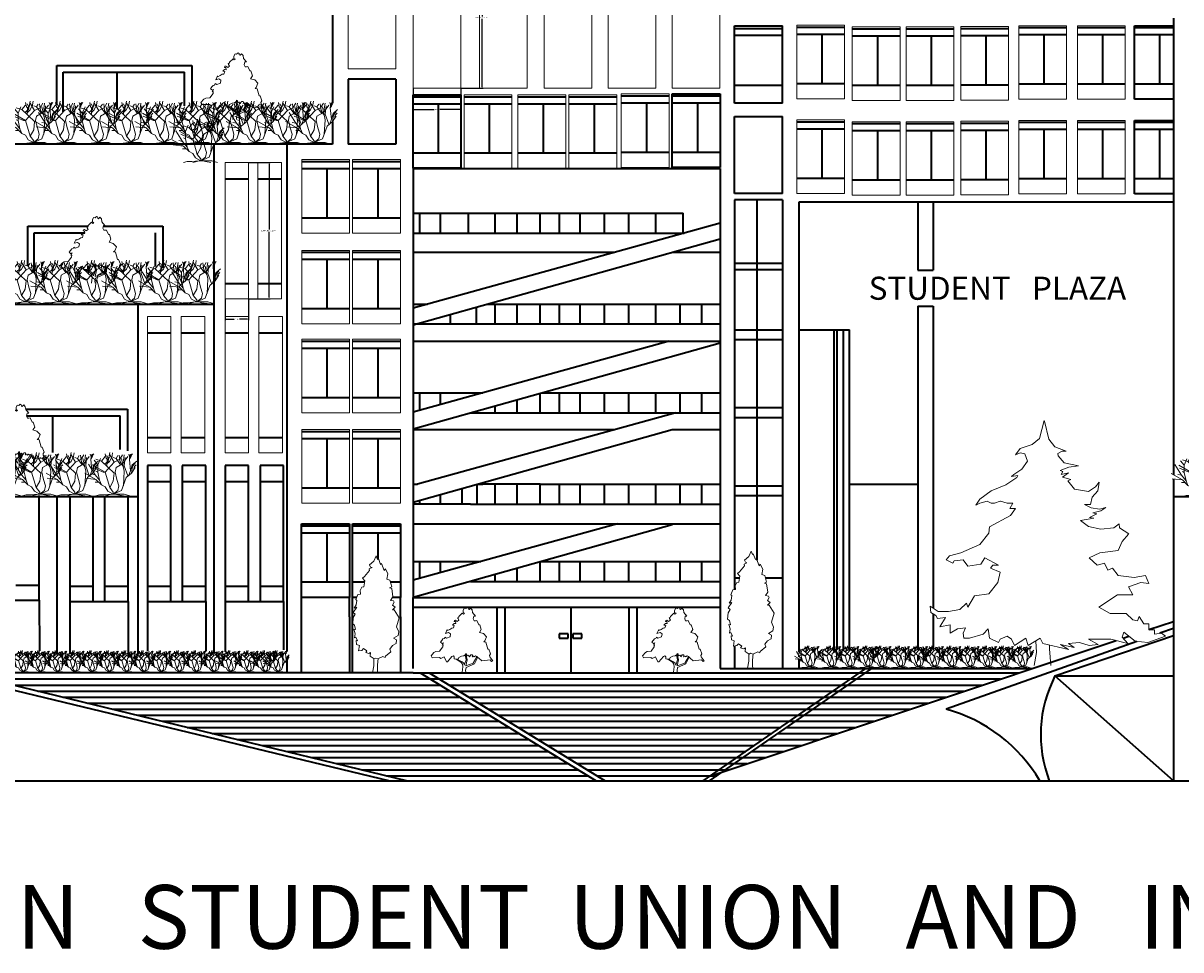
# Model space of a CAD drawing. Units: inches. Extents: x -362 to 223, y -437 to 70.
# Tile 3 of 5: x -124 to 67, y -166 to -13. Entities that reach past the tile are written whole.
import ezdxf

# ---------------------------------------------------------------- set-up
doc = ezdxf.new("R2010")
doc.units = ezdxf.units.IN
doc.header["$MEASUREMENT"] = 0
for name, color, linetype, lineweight in [('A-ANNO-DIMS', 2, 'Continuous', 18), ('A-ANNO-TEXT', 7, 'Continuous', 25), ('A-ELEV', 7, 'Continuous', 35), ('A-GLAZ', 4, 'Continuous', 18), ('L-PLNT', 3, 'Continuous', 13)]:
    doc.layers.add(name, color=color, linetype=linetype, lineweight=lineweight)
doc.styles.get("Standard").update_dxf_attribs({"font": 'arial.ttf'})
doc.dimstyles.get("Standard").update_dxf_attribs({"dimtxt": 0.18, "dimasz": 0.18, "dimexe": 0.18, "dimexo": 0.0625, "dimgap": 0.09, "dimtad": 0, "dimtih": 1, "dimtoh": 1, "dimdec": 4, "dimzin": 0, "dimdsep": 46, "dimtxsty": 'Standard', "dimcen": 0.09, "dimadec": 0, "dimazin": 0, "dimtfac": 1, "dimtdec": 4, "dimtofl": 0, "dimtmove": 0, "dimatfit": 3, "dimfxl": 1, "dimtolj": 1, "dimtzin": 0, "dimarcsym": 0})

# ---------------------------------------------------------------- blocks, each defined once
blk = doc.blocks.new('*U2')
for points in [[(22.0124, 137.721), (18.5475, 141.5624), (15.5282, 138.2446), (13.8028, 139.3505), (13.3714, 142.1153), (11.2148, 143.2214), (8.1954, 140.4564), (4.7447, 141.0094), (2.1567, 136.0326), (2.1567, 131.6088), (5.6074, 129.9499), (3.0193, 128.2909), (0.4313, 130.5029), (-6.9015, 123.3141), (-6.9015, 121.6552), (-9.9208, 119.9963), (-9.0581, 118.3373), (-6.9015, 115.0195), (-10.7835, 112.2546), (-14.6656, 115.0195), (-16.8222, 114.4665), (-17.6849, 112.2546), (-14.6656, 111.7016), (-14.2342, 107.2778), (-17.6065, 107.8307), (-21.5669, 103.9599), (-17.2536, 103.4069), (-18.9789, 97.8771), (-22.8609, 97.3241), (-27.1743, 94.5593), (-32.3504, 91.7944), (-32.7817, 94.0063), (-36.6638, 85.7116), (-29.7624, 87.3705), (-25.449, 84.6056), (-26.743, 77.9699), (-34.507, 75.205), (-37.9578, 77.4169), (-39.2518, 74.099), (-42.2711, 73.5461), (-44.8592, 70.2282), (-47.8786, 66.3574), (-43.9965, 63.0395), (-41.4085, 64.6985), (-44.3346, 59.8898), (-42.2089, 60.1377), (-42.5159, 55.7849), (-49.6039, 46.4502), (-58.2307, 45.8972), (-62.1127, 43.6853), (-68.5828, 36.4966), (-65.9947, 32.0727), (-50.0352, 32.6257), (-47.0159, 30.4138), (-39.6831, 33.7317), (-34.507, 22.6721), (-32.3504, 22.6721), (-22.4296, 34.8376), (-19.4102, 36.4966), (-17.2536, 33.7317), (-17.2536, 29.8608), (-13.8028, 28.7549), (-9.0581, 28.7549), (-7.3328, 32.6257), (-1.7254, 35.3906), (3.8821, 35.9436), (6.4701, 38.1555), (6.9014, 38.7085), (8.1954, 41.4734), (9.9208, 40.3674), (11.2148, 35.9436), (14.2341, 37.6025), (15.0968, 36.4966), (15.9595, 33.7317), (18.9789, 38.7085), (21.9982, 38.7085), (23.2922, 36.4966), (21.9982, 34.2847), (25.4489, 35.3906), (26.743, 33.7317), (29.7623, 35.9436), (32.7817, 34.8376), (38.8204, 28.7549), (41.4084, 27.6489), (43.5651, 25.437), (61.6813, 27.0959), (65.132, 23.7781), (67.7201, 24.884), (60.8186, 33.7317), (60.3873, 37.0495), (62.544, 40.3674), (58.662, 50.874), (56.5053, 50.874), (52.1919, 66.3574), (47.8785, 66.9103), (50.4665, 69.1222), (53.9172, 77.9699), (47.0158, 85.1586), (38.3891, 87.9235), (42.2711, 94.0063)], [(42.2711, 94.0063), (38.8204, 104.5129), (36.6637, 104.5129), (32.3503, 113.9135), (29.7623, 113.3605), (26.743, 113.3605), (24.5862, 117.7844), (25.8802, 123.8671), (29.331, 123.8671), (22.8609, 131.6088), (21.9982, 137.6916)], [(-12.9401, 28.7549), (-2.588, 22.1191), (0.8626, 17.6953), (1.7253, 11.6125), (0, 0)], [(-9.9208, 28.2019), (0, 23.2251), (3.4507, 19.9072), (4.7447, 15.4834), (8.6267, 27.0959), (6.4701, 37.6025)], [(34.5071, 33.1787), (27.1743, 18.2483), (9.0581, 10.5066), (7.7641, 3.8708), (8.1954, 0)], [(8.1954, 40.3674), (11.2148, 27.6489), (8.1954, 13.8245), (24.5862, 19.9072), (32.7817, 34.2847)]]:
    blk.add_lwpolyline(points)
blk = doc.blocks.new('*U3')
blk.add_lwpolyline([(-2.754, 191.699), (-6.78, 182.851), (-13.682, 176.953), (-11.956, 173.266), (-9.656, 172.529), (-14.257, 170.317), (-13.682, 167.368), (-21.733, 157.783), (-25.184, 154.834), (-21.158, 150.41), (-21.733, 147.461), (-22.884, 140.825), (-26.334, 140.087), (-29.21, 134.926), (-28.635, 129.028), (-32.661, 128.291), (-36.111, 120.18), (-34.386, 118.706), (-35.536, 111.333), (-38.987, 106.171), (-34.386, 107.646), (-40.712, 98.798), (-37.261, 95.849), (-40.712, 90.688), (-41.287, 80.366), (-38.412, 78.154), (-36.686, 70.781), (-39.562, 71.518), (-37.261, 64.145), (-38.412, 57.509), (-36.111, 58.247), (-33.236, 52.348), (-35.536, 53.086), (-34.961, 46.45), (-30.36, 44.975), (-31.51, 36.128), (-26.334, 36.865), (-23.459, 39.814), (-18.283, 36.128), (-20.008, 33.178), (-14.832, 31.704), (-11.956, 33.178), (-12.531, 27.28), (-6.205, 22.856), (-3.905, 24.331), (0.121, 22.856), (8.173, 26.543), (11.624, 25.068), (12.199, 27.28), (21.4, 34.653), (19.675, 39.077), (23.701, 44.975), (30.027, 47.924), (30.602, 53.823), (25.426, 56.772), (32.903, 61.196), (34.053, 67.094), (30.602, 75.205), (34.628, 89.951), (26.576, 103.222), (23.701, 103.222), (28.302, 107.646), (23.701, 110.595), (26.576, 115.756), (25.426, 117.968), (20.825, 118.706), (24.276, 124.604), (22.551, 137.876), (19.1, 139.35), (22.551, 140.825), (19.675, 151.884), (14.499, 153.359), (16.224, 162.207), (12.199, 170.317), (10.473, 167.368), (5.872, 179.165), (4.147, 177.69), (0.696, 187.275), (-0.454, 185.8)], close=True)
for points in [[(-6.813, 23.669), (-6.813, 11.669), (-8.627, 0)], [(0.387, 23.669), (-0.576, 13.271), (-0.576, 3.686), (0, 0)]]:
    blk.add_lwpolyline(points)
blk = doc.blocks.new('*U4')
for p, q in [((-16.8, 16.32), (-18.72, 18.72)), ((-14.88, 18.24), (-17.76, 19.2)), ((-16.8, 16.32), (-15.36, 19.68)), ((-14.88, 18.24), (-12.96, 20.64)), ((-8.16, 12), (-14.88, 18.24)), ((-13.325, 16.724), (-11.433, 18.289)), ((-12.471, 19.775), (-12.898, 22.044)), ((-11.677, 19.071), (-12.471, 19.775)), ((-11.28, 19.619), (-12.104, 21.184)), ((-12.043, 15.628), (-11.921, 18.836)), ((-11.921, 18.836), (-10.64, 20.401)), ((-11.433, 18.289), (-10.457, 22.749)), ((-10.579, 18.054), (-9.846, 19.697)), ((-8.16, 17.76), (-10.56, 21.6)), ((-9.48, 19.775), (-8.992, 22.592)), ((-7.2, 19.68), (-8.64, 20.16)), ((-8.16, 17.76), (-5.28, 19.2)), ((-7.2, 19.68), (-6.24, 21.12)), ((-4.8, 16.32), (-7.2, 19.68)), ((-5.086, 17.741), (-5.513, 21.34)), ((-5.28, 19.2), (-3.84, 21.6)), ((-2.88, 12.96), (-4.32, 19.68)), ((-3.84, 16.8), (-0.96, 20.64)), ((-3.377, 18.602), (-2.888, 21.575)), ((-2.766, 16.802), (-3.377, 18.602)), ((-2.88, 15.84), (-2.4, 20.16)), ((-0.508, 21.888), (-0.081, 20.558)), ((-0.203, 19.149), (0.102, 21.34)), ((0.346, 13.203), (-0.203, 19.149)), ((-0.142, 19.384), (0.59, 20.401)), ((-0.02, 20.01), (0.896, 21.105)), ((0.041, 20.714), (1.384, 22.044)), ((0.102, 21.34), (0.835, 21.888)), ((1.323, 16.254), (3.642, 18.289)), ((-18.24, 11.04), (-21.755, 16.655)), ((-12.96, 12.48), (-19.68, 16.32)), ((-13.92, 12.48), (-19.2, 14.88)), ((-16.8, 12.48), (-17.76, 12.96)), ((-16.8, 12.48), (-16.8, 16.32)), ((-15.84, 8.16), (-16.8, 12.48)), ((-12.96, 12.48), (-13.92, 12.48)), ((-12.96, 12.48), (-8.16, 17.76)), ((-10.56, 4.32), (-12.96, 12.48)), ((-11.982, 16.802), (-10.579, 18.054)), ((-7.68, 12.48), (-7.2, 14.88)), ((-6.72, 8.64), (-7.68, 12.48)), ((-7.2, 14.88), (-3.84, 16.8)), ((-3.377, 15.315), (-5.086, 17.819)), ((-3.36, 5.28), (-2.88, 12.96)), ((-0.96, 10.56), (-2.88, 15.84)), ((-0.48, 10.8), (0.346, 13.203)), ((0.346, 13.203), (1.323, 16.254)), ((0.96, 12), (1.44, 15.36)), ((0.96, 12), (2.88, 14.88)), ((1.44, 15.36), (2.88, 17.28)), ((1.92, 13.44), (2.4, 15.36)), ((2.4, 15.36), (3.36, 16.32)), ((-17.76, 8.64), (-23.663, 11.961)), ((-17.76, 8.64), (-23.128, 9.222)), ((-18.24, 11.04), (-20.16, 11.52)), ((-15.84, 8.16), (-18.24, 11.04)), ((-16.32, 7.2), (-18.24, 7.2)), ((-14.88, 5.76), (-17.76, 8.64)), ((-14.88, 5.76), (-15.84, 8.16)), ((-10.56, 4.32), (-8.64, 7.68)), ((-8.64, 7.68), (-8.16, 12)), ((-5.76, 5.28), (-6.72, 8.64)), ((-4.32, 2.88), (-1.92, 9.6)), ((-1.92, 9.6), (0.96, 12)), ((-15.84, 0.48), (-17.76, 0)), ((-13.44, 0.48), (-15.84, 0.48)), ((-12.96, 4.8), (-14.88, 5.76)), ((-9.6, 0.96), (-13.44, 0.48)), ((-11.52, 2.4), (-12.96, 4.8)), ((-9.6, 0.96), (-12.96, 0)), ((-8.64, 0.96), (-11.52, 2.4)), ((-8.64, 1.92), (-10.56, 4.32)), ((-9.6, 0.96), (-7.68, 0.96)), ((-8.64, 0.96), (-4.32, 2.88)), ((-8.64, 0.96), (-6.24, 2.88)), ((-8.64, 0.96), (-8.64, 1.92)), ((-8.64, 0.96), (-2.88, 0.96)), ((-7.68, 0.96), (-6.24, 0.48)), ((-6.24, 2.88), (-5.76, 5.28)), ((-6.24, 0.48), (-3.36, 0)), ((-2.88, 0.96), (0, 0))]:
    blk.add_line(p, q)
blk = doc.blocks.new('*U5')
for p, q in [((-8.263, 7.598), (-8.747, 14.105)), ((-9.75, 0), (-8.263, 7.598)), ((-0.771, 9.56), (-0.69, 11.833)), ((0, 0), (-0.771, 9.56))]:
    blk.add_line(p, q)
for points in [[(-3.9, 142.35), (-6.596, 132.037), (-10.801, 128.443), (-17.81, 126.047), (-20.614, 122.452), (-17.81, 123.65), (-15.007, 123.051), (-13.605, 118.858), (-16.876, 114.065), (-21.549, 111.07), (-22.951, 109.872), (-19.212, 110.471), (-19.68, 109.273), (-26.222, 105.079), (-34.633, 101.485), (-41.175, 96.693), (-43.511, 93.098), (-41.175, 94.296), (-36.969, 95.494), (-34.633, 94.296), (-32.764, 94.296), (-29.493, 95.494)], [(-3.759, 141.97), (-1.074, 131.643), (2.437, 127.141), (8.84, 124.493), (6.568, 124.493), (4.09, 123.169), (4.296, 121.846), (7.807, 117.874), (16.069, 116.02), (10.492, 115.226), (5.535, 113.372), (6.981, 112.843), (5.948, 110.989), (10.286, 112.048), (6.775, 109.401), (11.732, 108.077), (9.873, 107.282), (13.797, 102.516), (21.852, 101.192), (25.983, 103.84), (28.048, 106.488), (27.842, 105.164), (27.429, 101.457), (24.124, 97.75), (23.091, 93.513), (19.58, 93.513), (23.505, 91.66), (28.255, 90.866), (31.973, 91.925), (29.081, 89.806), (24.537, 88.747), (26.809, 88.218), (22.472, 86.099), (24.95, 85.57), (17.308, 84.246), (21.852, 80.804), (29.081, 79.215), (36.723, 80.009), (39.821, 82.392), (40.028, 80.009), (45.398, 76.567)], [(-29.25, 95.55), (-25.287, 94.296), (-22.016, 94.296), (-23.885, 91.301), (-20.614, 91.301), (-23.418, 87.108), (-35.567, 80.518), (-36.035, 76.924), (-41.175, 70.334), (-52.389, 65.542), (-58.931, 63.744), (-60.8, 61.348), (-57.062, 59.551), (-56.128, 60.749), (-50.987, 61.348), (-48.184, 57.754), (-40.707, 58.952), (-38.371, 62.546), (-30.427, 58.353), (-33.698, 58.353), (-35.1, 56.556), (-29.493, 54.159), (-30.894, 48.169), (-36.035, 41.579), (-44.446, 40.381), (-48.184, 33.791), (-49.118, 36.188), (-52.857, 32.593), (-59.399, 31.395), (-65.473, 31.395), (-70.146, 34.39), (-69.679, 30.796), (-66.875, 28.999), (-65.941, 27.202), (-61.268, 27.801), (-64.539, 22.409), (-58.464, 23.607), (-58.464, 18.815), (-54.258, 21.211), (-49.586, 21.81), (-50.987, 18.815), (-50.52, 15.82), (-47.249, 15.82), (-39.306, 18.216), (-36.502, 21.211), (-35.567, 15.82), (-30.427, 13.423), (-29.493, 15.221), (-25.287, 17.018), (-22.951, 15.221), (-21.081, 11.626), (-14.539, 15.82), (-13.138, 11.626), (-6.128, 15.82), (-4.726, 12.824), (10.226, 9.23), (5.554, 12.225), (13.497, 10.428), (10.226, 12.824), (16.768, 13.423), (22.376, 11.626), (27.516, 12.225), (21.909, 15.221), (34.993, 15.221), (44.806, 12.824), (41.535, 16.419), (42.469, 19.414), (49.011, 14.023), (56.487, 13.423), (66.768, 17.018), (64.431, 18.815), (60.226, 18.216), (60.226, 20.612), (56.955, 20.612), (56.955, 24.206), (54.151, 24.206), (51.348, 28.4), (50.413, 26.004), (47.609, 26.603), (43.871, 30.197), (38.731, 30.197), (34.525, 30.197), (27.983, 33.791), (38.731, 40.98), (47.609, 40.98), (45.273, 45.773), (52.282, 48.169), (56.955, 47.57), (55.086, 52.362), (48.544, 51.164), (39.198, 52.362), (35.927, 56.556), (33.123, 55.357), (31.254, 59.551), (27.049, 58.353), (22.376, 62.546), (28.451, 65.542), (39.198, 66.74), (41.535, 72.131), (45.273, 76.325)]]:
    blk.add_lwpolyline(points)
blk = doc.blocks.new('WIN-PANEL-A')
for p, q in [((0, 12.16), (7.9, 12.16)), ((0, 0), (0, 12.16)), ((7.9, 12.16), (7.9, 0)), ((7.9, 0), (0, 0))]:
    blk.add_line(p, q)
blk = doc.blocks.new('WIN-B')
for p, q in [((0, 23.36), (7.9, 23.36)), ((0, 23.36), (0, 0)), ((0, 23.36), (7.9, 23.36)), ((7.9, 0), (7.9, 23.36)), ((0, 0), (7.9, 0))]:
    blk.add_line(p, q)
blk = doc.blocks.new('WIN-SLOT')
for p, q in [((3.88, 22.5), (0, 22.5)), ((0, 22.5), (0, 21.75)), ((0, 21.75), (0, 0)), ((3.88, 0), (3.88, 22.5)), ((0, 0), (3.88, 0))]:
    blk.add_line(p, q)
blk = doc.blocks.new('*D19')
at = {"layer": 'A-ANNO-DIMS', "color": 0, "lineweight": -2, "transparency": 16777216}
for p, q in [((-51.81, 0.04), (-48.19, 0.04)), ((-48.37, -0.14), (-48.37, -11.45)), ((-48.37, -23.13), (-48.37, -11.82)), ((-51.81, -23.31), (-48.19, -23.31))]:
    blk.add_line(p, q, dxfattribs=at)
at = {"layer": 'A-ANNO-DIMS', "color": 0, "transparency": 16777216}
for points in [[(-48.4, -0.14), (-48.34, -0.14), (-48.37, 0.04)], [(-48.4, -23.13), (-48.34, -23.13), (-48.37, -23.31)]]:
    blk.add_solid(points, dxfattribs=at)
at = {"layer": 'Defpoints', "color": 0, "transparency": 16777216}
for p in [(-51.87, 0.04), (-48.37, 0.04), (-51.87, -23.31)]:
    blk.add_point(p, dxfattribs=at)
at = {"layer": 'A-ANNO-DIMS', "color": 0, "transparency": 16777216, "insert": (-48.37, -11.63), "char_height": 0.18, "attachment_point": 5}
blk.add_mtext('\\A1;WINDOW B 23 TYP.', dxfattribs=at)
blk = doc.blocks.new('*D20')
at = {"layer": 'A-ANNO-DIMS', "color": 0, "lineweight": -2, "transparency": 16777216}
for p, q in [((-59.77, -23.38), (-59.77, -27)), ((-51.87, -23.38), (-51.87, -27)), ((-59.59, -26.82), (-56.28, -26.82)), ((-52.05, -26.82), (-55.36, -26.82))]:
    blk.add_line(p, q, dxfattribs=at)
at = {"layer": 'A-ANNO-DIMS', "color": 0, "transparency": 16777216}
for points in [[(-59.59, -26.79), (-59.59, -26.85), (-59.77, -26.82)], [(-52.05, -26.79), (-52.05, -26.85), (-51.87, -26.82)]]:
    blk.add_solid(points, dxfattribs=at)
at = {"layer": 'Defpoints', "color": 0, "transparency": 16777216}
for p in [(-59.77, -23.31), (-51.87, -23.31), (-51.87, -26.82)]:
    blk.add_point(p, dxfattribs=at)
at = {"layer": 'A-ANNO-DIMS', "color": 0, "transparency": 16777216, "insert": (-55.82, -26.82), "char_height": 0.18, "attachment_point": 5}
blk.add_mtext('\\A1;8 TYP.', dxfattribs=at)
blk = doc.blocks.new('*D23')
at = {"layer": 'A-ANNO-DIMS', "color": 0, "lineweight": -2, "transparency": 16777216}
for p, q in [((-86.93, -35.62), (-83.43, -35.62)), ((-83.61, -35.8), (-83.61, -46.68)), ((-83.61, -57.94), (-83.61, -47.05)), ((-86.93, -58.12), (-83.43, -58.12))]:
    blk.add_line(p, q, dxfattribs=at)
at = {"layer": 'A-ANNO-DIMS', "color": 0, "transparency": 16777216}
for points in [[(-83.64, -35.8), (-83.58, -35.8), (-83.61, -35.62)], [(-83.64, -57.94), (-83.58, -57.94), (-83.61, -58.12)]]:
    blk.add_solid(points, dxfattribs=at)
at = {"layer": 'Defpoints', "color": 0, "transparency": 16777216}
for p in [(-86.99, -35.62), (-83.61, -35.62), (-86.99, -58.12)]:
    blk.add_point(p, dxfattribs=at)
at = {"layer": 'A-ANNO-DIMS', "color": 0, "transparency": 16777216, "insert": (-83.61, -46.87), "char_height": 0.18, "attachment_point": 5}
blk.add_mtext('\\A1;SLOT WINDOW 23 TYP.', dxfattribs=at)
blk = doc.blocks.new('*D24')
at = {"layer": 'A-ANNO-DIMS', "color": 0, "lineweight": -2, "transparency": 16777216}
for p, q in [((-90.87, -58.18), (-90.87, -61.67)), ((-86.99, -58.18), (-86.99, -61.67)), ((-90.69, -61.49), (-89.39, -61.49)), ((-87.17, -61.49), (-88.47, -61.49))]:
    blk.add_line(p, q, dxfattribs=at)
at = {"layer": 'A-ANNO-DIMS', "color": 0, "transparency": 16777216}
for points in [[(-90.69, -61.46), (-90.69, -61.52), (-90.87, -61.49)], [(-87.17, -61.46), (-87.17, -61.52), (-86.99, -61.49)]]:
    blk.add_solid(points, dxfattribs=at)
at = {"layer": 'Defpoints', "color": 0, "transparency": 16777216}
for p in [(-90.87, -58.12), (-86.99, -58.12), (-86.99, -61.49)]:
    blk.add_point(p, dxfattribs=at)
at = {"layer": 'A-ANNO-DIMS', "color": 0, "transparency": 16777216, "insert": (-88.93, -61.49), "char_height": 0.18, "attachment_point": 5}
blk.add_mtext('\\A1;4 TYP.', dxfattribs=at)

msp = doc.modelspace()

# ---------------------------------------------------------------- linework, layer by layer
at = {"layer": 'A-ELEV'}
for p, q in [((-73.12, -6.5), (-73.12, -25.79)), ((-6.6, -25.76), (-6.6, -12.99)), ((-6.6, -12.99), (1.3, -12.99)), ((1.3, -25.76), (1.3, -12.99)), ((3.69, -13.23), (11.59, -13.23)), ((40.39, -13.29), (48.29, -13.29)), ((50.11, -13.29), (58.01, -13.29)), ((59.56, -12.97), (65.97, -12.97)), ((59.56, -25.13), (59.56, -12.97)), ((59.56, -13.29), (65.97, -13.29)), ((65.97, -11.74), (65.97, -58.78)), ((-6.6, -13.45), (1.3, -13.45)), ((-6.6, -14.52), (1.3, -14.52)), ((3.69, -14.38), (11.59, -14.38)), ((7.9, -22.53), (7.9, -14.38)), ((12.87, -13.5), (20.77, -13.5)), ((12.87, -14.66), (20.77, -14.66)), ((17.07, -22.8), (17.07, -14.66)), ((21.77, -13.5), (29.67, -13.5)), ((21.77, -14.66), (29.67, -14.66)), ((25.97, -22.8), (25.97, -14.66)), ((30.8, -13.43), (38.7, -13.43)), ((30.8, -14.58), (38.7, -14.58)), ((35.01, -22.73), (35.01, -14.58)), ((40.39, -14.45), (48.29, -14.45)), ((44.59, -22.59), (44.59, -14.45)), ((50.11, -14.45), (58.01, -14.45)), ((54.31, -22.59), (54.31, -14.45)), ((59.56, -14.45), (65.97, -14.45)), ((63.76, -22.59), (63.76, -14.45)), ((-118.69, -26.06), (-118.69, -19.58)), ((-118.69, -19.58), (-96.36, -19.58)), ((-117.66, -20.67), (-97.57, -20.67)), ((-117.66, -27.21), (-117.66, -20.67)), ((-108.73, -26.72), (-108.73, -20.67)), ((-97.57, -26.24), (-97.57, -20.67)), ((-96.36, -19.58), (-96.36, -26.45)), ((-62.63, -21.79), (-70.53, -21.79)), ((-70.53, -21.79), (-70.53, -32.58)), ((-62.63, -21.79), (-62.63, -32.58)), ((-6.6, -22.82), (1.3, -22.82)), ((3.69, -22.53), (11.59, -22.53)), ((12.87, -22.8), (20.77, -22.8)), ((21.77, -22.8), (29.67, -22.8)), ((30.8, -22.73), (38.7, -22.73)), ((40.39, -22.59), (48.29, -22.59)), ((50.11, -22.59), (58.01, -22.59)), ((59.56, -22.59), (65.97, -22.59)), ((-59.78, -24.4), (-51.88, -24.4)), ((-59.78, -36.56), (-59.78, -24.4)), ((-59.78, -24.72), (-51.88, -24.72)), ((-51.88, -24.4), (-51.88, -36.56)), ((-51.35, -24.72), (-43.45, -24.72)), ((-42.43, -24.72), (-34.53, -24.72)), ((-34.01, -24.72), (-26.1, -24.72)), ((-25.34, -24.59), (-17.44, -24.59)), ((-16.92, -24.27), (-9.01, -24.27)), ((-16.92, -36.43), (-16.92, -24.27)), ((-16.92, -24.59), (-9.01, -24.59)), ((-9.01, -24.27), (-9.01, -36.43)), ((-59.78, -25.88), (-51.88, -25.88)), ((-55.58, -34.02), (-55.58, -25.88)), ((-51.35, -25.88), (-43.45, -25.88)), ((-47.15, -34.02), (-47.15, -25.88)), ((-42.43, -25.88), (-34.53, -25.88)), ((-38.23, -34.02), (-38.23, -25.88)), ((-34.01, -25.88), (-26.1, -25.88)), ((-29.8, -34.02), (-29.8, -25.88)), ((-25.34, -25.75), (-17.44, -25.75)), ((-21.14, -33.9), (-21.14, -25.75)), ((-16.92, -25.75), (-9.01, -25.75)), ((-12.71, -33.9), (-12.71, -25.75)), ((1.3, -25.76), (-6.6, -25.76)), ((65.97, -25.13), (59.56, -25.13)), ((-6.6, -40.73), (-6.6, -27.97)), ((-6.6, -27.97), (1.3, -27.97)), ((1.3, -40.73), (1.3, -27.97)), ((59.56, -28.64), (65.97, -28.64)), ((59.56, -40.8), (59.56, -28.64)), ((-73.12, -28.82), (-73.12, -32.58)), ((3.69, -28.89), (11.59, -28.89)), ((3.69, -30.05), (11.59, -30.05)), ((7.9, -38.2), (7.9, -30.05)), ((12.87, -29.16), (20.77, -29.16)), ((12.87, -30.32), (20.77, -30.32)), ((17.07, -38.47), (17.07, -30.32)), ((21.77, -29.16), (29.67, -29.16)), ((21.77, -30.32), (29.67, -30.32)), ((25.97, -38.47), (25.97, -30.32)), ((30.8, -29.09), (38.7, -29.09)), ((30.8, -30.25), (38.7, -30.25)), ((35.01, -38.4), (35.01, -30.25)), ((40.39, -28.95), (48.29, -28.95)), ((40.39, -30.11), (48.29, -30.11)), ((44.59, -38.26), (44.59, -30.11)), ((50.11, -28.95), (58.01, -28.95)), ((50.11, -30.11), (58.01, -30.11)), ((54.31, -38.26), (54.31, -30.11)), ((59.56, -28.95), (65.97, -28.95)), ((59.56, -30.11), (65.97, -30.11)), ((63.76, -38.26), (63.76, -30.11)), ((-80.64, -32.58), (-183.41, -32.58)), ((-92.76, -32.58), (-92.76, -116.73)), ((-73.12, -32.58), (-87.17, -32.58)), ((-80.64, -32.58), (-80.64, -59)), ((-62.63, -32.58), (-70.53, -32.58)), ((-59.78, -34.02), (-51.88, -34.02)), ((-51.35, -34.02), (-43.45, -34.02)), ((-42.43, -34.02), (-34.53, -34.02)), ((-34.01, -34.02), (-26.1, -34.02)), ((-25.34, -33.9), (-17.44, -33.9)), ((-16.92, -33.9), (-9.01, -33.9)), ((-78.22, -35.44), (-70.31, -35.44)), ((-69.79, -35.44), (-61.89, -35.44)), ((-78.22, -36.6), (-70.31, -36.6)), ((-74.01, -44.75), (-74.01, -36.6)), ((-69.79, -36.6), (-61.89, -36.6)), ((-65.58, -44.75), (-65.58, -36.6)), ((-51.88, -36.56), (-59.78, -36.56)), ((-59.77, -36.6), (-9, -36.6)), ((-59.77, -36.6), (-59.77, -107.51)), ((-9.01, -36.43), (-16.92, -36.43)), ((-16.92, -36.43), (-16.92, -36.6)), ((-9, -36.6), (-9, -107.51)), ((3.69, -38.2), (11.59, -38.2)), ((40.39, -38.26), (48.29, -38.26)), ((50.11, -38.26), (58.01, -38.26)), ((59.56, -38.26), (65.97, -38.26)), ((-90.87, -38.3), (-86.99, -38.3)), ((-85.45, -38.3), (-81.57, -38.3)), ((12.87, -38.47), (20.77, -38.47)), ((21.77, -38.47), (29.67, -38.47)), ((30.8, -38.4), (38.7, -38.4)), ((1.3, -40.73), (-6.6, -40.73)), ((1.3, -41.75), (-6.6, -41.75)), ((-6.6, -41.75), (-6.6, -104.27)), ((-2.89, -101.37), (-2.89, -41.75)), ((1.3, -41.75), (1.3, -119.3)), ((65.97, -40.8), (59.56, -40.8)), ((-59.77, -43.97), (-47.8, -43.97)), ((-58.68, -47.28), (-58.68, -43.97)), ((-55.22, -43.97), (-15.09, -43.97)), ((-55.22, -47.28), (-55.22, -43.97)), ((-50.59, -47.28), (-50.59, -43.97)), ((-46.21, -47.28), (-46.21, -43.97)), ((-42.55, -47.28), (-42.55, -43.97)), ((-38.76, -47.28), (-38.76, -43.97)), ((-35.56, -47.28), (-35.56, -43.97)), ((-32.16, -47.28), (-32.16, -43.97)), ((-28.11, -47.28), (-28.11, -43.97)), ((-24.12, -47.28), (-24.12, -43.97)), ((-19.62, -47.28), (-19.62, -43.97)), ((-15.09, -47.28), (-15.09, -43.97)), ((65.97, -42.14), (4.03, -42.14)), ((4.03, -42.14), (4.03, -116.57)), ((23.71, -42.14), (23.71, -53.43)), ((26.23, -42.14), (26.23, -53.43)), ((-78.22, -44.75), (-70.31, -44.75)), ((-69.79, -44.75), (-61.89, -44.75)), ((-9, -45.63), (-59.77, -59.66)), ((-123.51, -52.61), (-123.51, -46.12)), ((-123.51, -46.12), (-113.53, -46.12)), ((-122.48, -47.21), (-114.1, -47.21)), ((-122.48, -53.75), (-122.48, -47.21)), ((-111.03, -46.12), (-101.18, -46.12)), ((-102.39, -52.78), (-102.39, -47.21)), ((-101.18, -46.12), (-101.18, -52.99)), ((-59.77, -47.28), (-14.97, -47.28)), ((-49.85, -47.28), (-14.97, -47.28)), ((-59.77, -62.44), (-9, -48.23)), ((-78.22, -50.44), (-70.31, -50.44)), ((-78.22, -51.6), (-70.31, -51.6)), ((-74.01, -59.75), (-74.01, -51.6)), ((-69.79, -50.44), (-61.89, -50.44)), ((-69.79, -51.6), (-61.89, -51.6)), ((-65.58, -59.75), (-65.58, -51.6)), ((-59.77, -50.44), (-26.41, -50.44)), ((-16.92, -50.44), (-9, -50.44)), ((-113.55, -53.26), (-113.55, -52.73)), ((-6.6, -52.23), (1.3, -52.23)), ((-6.6, -53.32), (1.3, -53.32)), ((23.71, -53.43), (26.23, -53.43)), ((-90.87, -55.62), (-86.99, -55.62)), ((-85.45, -55.62), (-81.57, -55.62)), ((-219.64, -59), (-92.76, -59)), ((-105.32, -59), (-105.32, -116.96)), ((-80.64, -59), (-80.64, -116.43)), ((-59.77, -59), (-57.38, -59)), ((-58.68, -59.36), (-58.68, -59)), ((-47.48, -59), (-9, -59)), ((-46.21, -62.32), (-46.21, -59)), ((-42.55, -62.32), (-42.55, -59)), ((-38.76, -62.32), (-38.76, -59)), ((-35.56, -62.32), (-35.56, -59)), ((-32.16, -62.32), (-32.16, -59)), ((-28.11, -62.32), (-28.11, -59)), ((-24.12, -62.32), (-24.12, -59)), ((-19.62, -62.32), (-19.62, -59)), ((-15.63, -62.32), (-15.63, -59)), ((-12.04, -62.32), (-12.04, -59)), ((23.71, -59.35), (23.71, -116.18)), ((23.71, -59.35), (26.23, -59.35)), ((26.23, -59.35), (26.23, -109.29)), ((65.97, -58.78), (65.97, -87.25)), ((-78.22, -59.75), (-70.31, -59.75)), ((-69.79, -59.75), (-61.89, -59.75)), ((-53.6, -62.28), (-53.6, -60.72)), ((-49.29, -62.28), (-49.29, -59.51)), ((-59.77, -62.28), (-9, -62.28)), ((-103.72, -63.77), (-99.84, -63.77)), ((-98.12, -63.77), (-94.24, -63.77)), ((-90.87, -63.77), (-86.99, -63.77)), ((-85.28, -63.77), (-81.4, -63.77)), ((-6.6, -63.26), (1.3, -63.26)), ((-6.6, -64.88), (1.3, -64.88)), ((4.03, -63.26), (12.39, -63.26)), ((9.89, -116.18), (9.89, -63.26)), ((10.39, -116.08), (10.39, -63.26)), ((11.39, -116.26), (11.39, -63.26)), ((11.39, -116.26), (11.39, -63.26)), ((12.39, -116.36), (12.39, -63.26)), ((-78.22, -65.15), (-70.31, -65.15)), ((-78.22, -66.31), (-70.31, -66.31)), ((-74.01, -74.46), (-74.01, -66.31)), ((-69.79, -65.15), (-61.89, -65.15)), ((-69.79, -66.31), (-61.89, -66.31)), ((-65.58, -74.46), (-65.58, -66.31)), ((-59.77, -65.15), (-9, -65.15)), ((-17.4, -65.15), (-59.77, -76.86)), ((-59.77, -79.64), (-9, -65.43)), ((-78.22, -74.46), (-70.31, -74.46)), ((-69.79, -74.46), (-61.89, -74.46)), ((-59.77, -73.68), (-48.26, -73.68)), ((-58.68, -76.55), (-58.68, -73.68)), ((-55.22, -75.6), (-55.22, -73.68)), ((-38.76, -76.99), (-38.76, -73.76)), ((-38.48, -73.68), (-9, -73.68)), ((-35.56, -76.99), (-35.56, -73.68)), ((-32.16, -76.99), (-32.16, -73.68)), ((-28.11, -76.99), (-28.11, -73.68)), ((-24.12, -76.99), (-24.12, -73.68)), ((-19.62, -76.99), (-19.62, -73.68)), ((-15.63, -76.99), (-15.63, -73.68)), ((-12.04, -76.99), (-12.04, -73.68)), ((-123.87, -76.41), (-107, -76.41)), ((-107, -76.41), (-107, -83.29)), ((-46.21, -76.99), (-46.21, -75.84)), ((-42.55, -76.99), (-42.55, -74.82)), ((-6.6, -76.12), (1.3, -76.12)), ((-123.73, -77.5), (-108.21, -77.5)), ((-119.36, -83.55), (-119.36, -77.5)), ((-108.21, -83.07), (-108.21, -77.5)), ((-16.34, -76.99), (-59.04, -88.79)), ((-50.31, -76.99), (-9, -76.99)), ((-6.6, -77.75), (1.3, -77.75)), ((-78.22, -80.09), (-70.31, -80.09)), ((-69.79, -80.09), (-61.89, -80.09)), ((-59.77, -79.78), (-26.41, -79.78)), ((-59.77, -91.77), (-16.92, -79.78)), ((-16.92, -79.78), (-9, -79.78)), ((-103.72, -81.09), (-99.84, -81.09)), ((-98.12, -81.09), (-94.24, -81.09)), ((-90.87, -81.09), (-86.99, -81.09)), ((-85.28, -81.09), (-81.4, -81.09)), ((-78.22, -81.25), (-70.31, -81.25)), ((-74.01, -89.4), (-74.01, -81.25)), ((-69.79, -81.25), (-61.89, -81.25)), ((-65.58, -89.4), (-65.58, -81.25)), ((-99.84, -85.68), (-103.72, -85.68)), ((-103.72, -85.68), (-103.72, -86.43)), ((-99.84, -108.18), (-99.84, -85.68)), ((-94.07, -85.68), (-97.95, -85.68)), ((-97.95, -85.68), (-97.95, -86.43)), ((-94.07, -108.18), (-94.07, -85.68)), ((-86.99, -85.68), (-90.87, -85.68)), ((-90.87, -85.68), (-90.87, -86.43)), ((-86.99, -108.18), (-86.99, -85.68)), ((-81.22, -85.68), (-85.1, -85.68)), ((-85.1, -85.68), (-85.1, -86.43)), ((-81.22, -108.18), (-81.22, -85.68)), ((-103.72, -86.43), (-103.72, -108.18)), ((-97.95, -86.43), (-97.95, -108.18)), ((-90.87, -86.43), (-90.87, -108.18)), ((-85.1, -86.43), (-85.1, -108.18)), ((65.97, -87.93), (65.97, -90.83)), ((-103.72, -88.37), (-99.84, -88.37)), ((-97.95, -88.37), (-94.07, -88.37)), ((-90.87, -88.37), (-86.99, -88.37)), ((-85.1, -88.37), (-81.22, -88.37)), ((-78.22, -89.4), (-70.31, -89.4)), ((-69.79, -89.4), (-61.89, -89.4)), ((-59.77, -88.79), (-59.04, -88.79)), ((-51.65, -92.1), (-51.65, -89.5)), ((-49.18, -92.1), (-49.18, -88.79)), ((-49.18, -88.79), (-48.26, -88.79)), ((-38.76, -88.79), (-48.26, -88.79)), ((-46.21, -92.1), (-46.21, -88.79)), ((-42.55, -92.1), (-42.55, -88.79)), ((-38.76, -88.79), (-9, -88.79)), ((-38.76, -92.1), (-38.76, -88.79)), ((-35.56, -92.1), (-35.56, -88.79)), ((-32.16, -92.1), (-32.16, -88.79)), ((-28.11, -92.1), (-28.11, -88.79)), ((-24.12, -92.1), (-24.12, -88.79)), ((-19.62, -92.1), (-19.62, -88.79)), ((-15.63, -92.1), (-15.63, -88.79)), ((-12.04, -92.1), (-12.04, -88.79)), ((-6.6, -89.05), (1.3, -89.05)), ((12.39, -88.79), (23.71, -88.79)), ((-248.18, -90.83), (-105.32, -90.83)), ((-121.61, -108), (-121.61, -90.65)), ((-118.7, -90.83), (-118.7, -116.92)), ((-116.57, -90.83), (-116.57, -108.18)), ((-112.69, -108.18), (-112.69, -90.83)), ((-110.8, -90.83), (-110.8, -108.18)), ((-106.92, -108.18), (-106.92, -90.83)), ((-58.68, -92.1), (-58.68, -91.47)), ((-55.22, -92.1), (-55.22, -90.5)), ((-6.6, -90.68), (1.3, -90.68)), ((65.97, -90.83), (119.87, -90.83)), ((65.97, -90.83), (65.97, -137.85)), ((-50.31, -92.1), (-59.77, -92.1)), ((-50.31, -92.1), (-9, -92.1)), ((-78.22, -95.35), (-70.31, -95.35)), ((-78.22, -107.51), (-78.22, -95.35)), ((-78.22, -95.67), (-70.31, -95.67)), ((-70.31, -95.35), (-70.31, -107.51)), ((-69.79, -95.35), (-61.89, -95.35)), ((-69.79, -107.51), (-69.79, -95.35)), ((-69.79, -95.67), (-61.89, -95.67)), ((-61.89, -95.35), (-61.89, -107.51)), ((-59.77, -95.35), (-9, -95.35)), ((-25.98, -95.35), (-59.77, -104.69)), ((-59.77, -107.47), (-16.92, -95.47)), ((-78.22, -96.82), (-70.31, -96.82)), ((-74.01, -104.97), (-74.01, -96.82)), ((-69.79, -96.82), (-61.89, -96.82)), ((-65.58, -101.15), (-65.58, -96.82)), ((-59.77, -101.59), (-48.58, -101.59)), ((-58.68, -104.46), (-58.68, -101.59)), ((-55.22, -103.52), (-55.22, -101.59)), ((-42.55, -104.91), (-42.55, -102.73)), ((-38.76, -101.59), (-9, -101.59)), ((-38.76, -104.91), (-38.76, -101.59)), ((-35.56, -104.91), (-35.56, -101.59)), ((-32.16, -104.91), (-32.16, -101.59)), ((-28.11, -104.91), (-28.11, -101.59)), ((-24.12, -104.91), (-24.12, -101.59)), ((-19.62, -104.91), (-19.62, -101.59)), ((-15.63, -104.91), (-15.63, -101.59)), ((-12.04, -104.91), (-12.04, -101.59)), ((-78.22, -104.97), (-70.31, -104.97)), ((-69.79, -104.97), (-67.77, -104.97)), ((-63.53, -104.97), (-61.89, -104.97)), ((-50.31, -104.91), (-9, -104.91)), ((-46.21, -104.91), (-46.21, -103.76)), ((-6.6, -104.27), (-5.76, -104.27)), ((-6.6, -104.27), (-6.6, -106.21)), ((-1.49, -104.27), (1.3, -104.27)), ((-125.49, -105.5), (-121.61, -105.5)), ((-116.57, -105.68), (-112.69, -105.68)), ((-110.8, -105.68), (-106.92, -105.68)), ((-103.72, -105.68), (-99.84, -105.68)), ((-97.95, -105.68), (-94.07, -105.68)), ((-90.87, -105.68), (-86.99, -105.68)), ((-85.1, -105.68), (-81.22, -105.68)), ((-181.3, -108.59), (-60.7, -137.85)), ((-131.26, -108), (-121.61, -108)), ((-125.49, -108), (-121.61, -108)), ((-121.61, -108), (-121.6, -116.33)), ((-116.57, -108.18), (-112.69, -108.18)), ((-116.57, -108.18), (-106.92, -108.18)), ((-116.57, -108.18), (-116.57, -116.92)), ((-110.8, -108.18), (-106.92, -108.18)), ((-106.92, -108.18), (-106.92, -117.34)), ((-103.72, -108.18), (-99.84, -108.18)), ((-103.72, -108.18), (-94.07, -108.18)), ((-103.72, -108.18), (-103.72, -116.34)), ((-97.95, -108.18), (-94.07, -108.18)), ((-94.07, -108.18), (-94.07, -116.41)), ((-90.87, -108.18), (-86.99, -108.18)), ((-90.87, -108.18), (-81.22, -108.18)), ((-90.87, -108.18), (-90.87, -116.53)), ((-85.1, -108.18), (-81.22, -108.18)), ((-81.22, -108.18), (-81.22, -116.17)), ((-70.31, -107.51), (-78.22, -107.51)), ((-78.22, -110.73), (-78.22, -107.51)), ((-70.31, -110.73), (-70.31, -107.51)), ((-69.79, -110.73), (-69.79, -107.51)), ((-69.1, -107.51), (-69.79, -107.51)), ((-61.89, -107.51), (-63.2, -107.51)), ((-61.89, -110.73), (-61.89, -107.51)), ((-59.77, -107.51), (-9, -107.51)), ((-59.77, -119.3), (-59.77, -107.51)), ((-9, -107.51), (-9, -119.3)), ((-181.11, -109.51), (-63.64, -137.85)), ((-78.22, -120.01), (-78.22, -110.73)), ((-70.31, -110.73), (-70.31, -120.01)), ((-69.79, -120.01), (-69.79, -110.73)), ((-61.89, -110.73), (-61.89, -120.01)), ((-59.77, -109.16), (-9, -109.16)), ((-45.95, -109.16), (-45.95, -120.01)), ((-44.63, -109.16), (-44.63, -120.01)), ((-33.69, -109.16), (-33.69, -120.01)), ((-24.08, -109.16), (-24.08, -120.01)), ((-22.75, -109.16), (-22.75, -120.01)), ((26.23, -110.23), (26.23, -116)), ((61.9, -112.84), (65.97, -111.49)), ((65.97, -112.66), (63.72, -113.46)), ((-35.62, -113.53), (-35.62, -114.24)), ((-34.15, -113.53), (-35.62, -113.53)), ((-35.62, -114.24), (-34.15, -114.24)), ((-34.15, -114.24), (-34.15, -113.53)), ((-33.36, -113.53), (-33.36, -114.24)), ((-31.89, -113.53), (-33.36, -113.53)), ((-33.36, -114.24), (-31.89, -114.24)), ((-31.89, -114.24), (-31.89, -113.53)), ((-10.56, -137.01), (56.5, -114.64)), ((59.94, -114.8), (28.39, -126.01)), ((46.39, -120.51), (65.97, -113.83)), ((57.66, -114.26), (58.62, -113.94)), ((-6.6, -115.55), (-6.6, -119.3)), ((9.89, -116.59), (9.89, -116.45)), ((10.39, -116.97), (10.39, -116.71)), ((-80.64, -117.96), (-80.64, -120.01)), ((4.03, -117.12), (4.03, -117.35)), ((4.03, -117.75), (4.03, -119.3)), ((10.39, -117.72), (10.39, -117.49)), ((11.39, -117.1), (11.39, -117)), ((11.39, -117.1), (11.39, -117)), ((23.71, -117.16), (23.71, -117.93)), ((26.23, -118.72), (26.23, -119.01)), ((-61.89, -120.01), (-134.22, -120.01)), ((-59.77, -120.01), (-61.89, -120.01)), ((-59.77, -120.01), (-58.6, -120.01)), ((-58.6, -120.01), (-29.5, -137.85)), ((-58.6, -120.01), (14.04, -120.01)), ((-57.1, -120.01), (-28, -137.85)), ((-11.78, -137.85), (15.08, -119.3)), ((-10.78, -137.85), (16.08, -119.3)), ((-9, -119.3), (15.08, -119.3)), ((-9, -119.3), (16.08, -119.3)), ((9.89, -119.3), (9.89, -119.01)), ((10.39, -119.3), (10.39, -119.06)), ((11.39, -119.3), (11.39, -119.09)), ((11.39, -119.3), (11.39, -119.09)), ((12.39, -119.01), (12.39, -118.99)), ((14.04, -120.01), (40.4, -120.01)), ((15.08, -119.3), (42.55, -119.3)), ((16.08, -119.3), (42.55, -119.3)), ((23.71, -118.86), (23.71, -119.01)), ((65.97, -137.85), (46.39, -120.51)), ((46.39, -120.51), (65.97, -120.51)), ((-130.1, -121.01), (-55.47, -121.01)), ((-125.98, -122.01), (-55.34, -122.01)), ((-55.47, -121.01), (12.6, -121.01)), ((-53.84, -122.01), (11.15, -122.01)), ((11.15, -122.01), (34.41, -122.01)), ((12.6, -121.01), (37.4, -121.01)), ((-121.85, -123.01), (-53.71, -123.01)), ((-117.73, -124.01), (-52.08, -124.01)), ((-52.21, -123.01), (9.7, -123.01)), ((-50.58, -124.01), (8.25, -124.01)), ((8.25, -124.01), (28.41, -124.01)), ((9.7, -123.01), (31.41, -123.01)), ((-113.61, -125.01), (-50.45, -125.01)), ((-109.49, -126.01), (-48.82, -126.01)), ((-48.95, -125.01), (6.81, -125.01)), ((-47.32, -126.01), (5.36, -126.01)), ((5.36, -126.01), (22.41, -126.01)), ((6.81, -125.01), (25.41, -125.01)), ((-105.37, -127.01), (-47.18, -127.01)), ((-101.25, -128.01), (-45.55, -128.01)), ((-45.68, -127.01), (3.91, -127.01)), ((-44.05, -128.01), (2.46, -128.01)), ((2.46, -128.01), (16.42, -128.01)), ((3.91, -127.01), (19.42, -127.01)), ((-97.13, -129.01), (-43.92, -129.01)), ((-93.01, -130.01), (-42.29, -130.01)), ((-42.42, -129.01), (1.02, -129.01)), ((-40.79, -130.01), (-0.43, -130.01)), ((0.57, -130.01), (10.42, -130.01)), ((2.02, -129.01), (13.42, -129.01)), ((-88.88, -131.01), (-40.66, -131.01)), ((-84.76, -132.01), (-39.03, -132.01)), ((-39.16, -131.01), (-1.88, -131.01)), ((-37.53, -132.01), (-3.33, -132.01)), ((-2.33, -132.01), (4.43, -132.01)), ((-0.88, -131.01), (7.42, -131.01)), ((-80.64, -133.01), (-37.4, -133.01)), ((-76.52, -134.01), (-35.76, -134.01)), ((-35.9, -133.01), (-4.77, -133.01)), ((-34.26, -134.01), (-6.22, -134.01)), ((-6.22, -134.01), (-1.57, -134.01)), ((-3.77, -133.01), (1.43, -133.01)), ((-72.4, -135.01), (-34.13, -135.01)), ((-32.63, -135.01), (-7.67, -135.01)), ((-7.67, -135.01), (-4.57, -135.01)), ((-188.3, -137.85), (-28, -137.85)), ((-68.28, -136.01), (-32.5, -136.01)), ((-64.16, -137.01), (-30.87, -137.01)), ((-31, -136.01), (-9.12, -136.01)), ((-29.37, -137.01), (-10.56, -137.01)), ((-28, -137.85), (-10.78, -137.85)), ((-11.78, -137.85), (200.92, -137.85)), ((-10.56, -137.01), (-9.56, -137.01)), ((-9.12, -136.01), (-7.57, -136.01)), ((65.97, -137.85), (119.87, -137.85))]:
    msp.add_line(p, q, dxfattribs=at)
for centre, radius, start, end in [((65.17, -130.22), 21.14, 152.6585, 201.1534), ((21.68, -150.83), 25.71, 30.3202, 74.8691)]:
    msp.add_arc(centre, radius, start, end, dxfattribs=at)

# ---------------------------------------------------------------- block references
at = {"layer": 'A-GLAZ'}
for name, p in [('WIN-B', (-59.77, -23.31)), ('WIN-B', (-48.8, -23.31)), ('WIN-B', (-38.09, -23.31)), ('WIN-B', (-27.52, -23.31)), ('WIN-B', (-16.94, -23.31)), ('WIN-SLOT', (-90.87, -58.12)), ('WIN-SLOT', (-85.45, -58.12)), ('WIN-SLOT', (-103.72, -83.59)), ('WIN-SLOT', (-98.12, -83.59)), ('WIN-SLOT', (-90.87, -83.59)), ('WIN-SLOT', (-85.28, -83.59))]:
    msp.add_blockref(name, p, dxfattribs=at)
at = {"layer": 'A-GLAZ', "rotation": 180}
for p in [(-62.63, -7.93), (11.59, -12.91), (20.77, -13.18), (29.67, -13.18), (38.7, -13.11), (48.29, -12.97), (58.01, -12.97), (-43.45, -24.4), (-34.53, -24.4), (-26.1, -24.4), (-17.44, -24.27), (11.59, -28.57), (48.29, -28.64), (58.01, -28.64), (20.77, -28.85), (29.67, -28.85), (38.7, -28.77), (-70.31, -35.12), (-61.89, -35.12), (-70.31, -50.13), (-61.89, -50.13), (-70.31, -64.83), (-61.89, -64.83), (-70.31, -79.78), (-61.89, -79.78)]:
    msp.add_blockref('WIN-PANEL-A', p, dxfattribs=at)
at = {"layer": 'L-PLNT'}
for name, p, xscale, yscale, zscale in [('*U2', (-89.6, -28.5), 0.0769249465327344, 0.0769249465327344, 0.0769249465327344), ('*U4', (-119.81, -32.6), 0.3151431067188808, 0.3151431067188808, 0.3151431067188808), ('*U4', (-114.86, -32.6), 0.3151431067188808, 0.3151431067188808, 0.3151431067188808), ('*U4', (-109.2, -32.6), 0.3151431067188808, 0.3151431067188808, 0.3151431067188808), ('*U4', (-103.88, -32.6), 0.3151431067188808, 0.3151431067188808, 0.3151431067188808), ('*U4', (-98.35, -32.6), 0.3151431067188808, 0.3151431067188808, 0.3151431067188808), ('*U4', (-92.73, -32.6), 0.3151431067188808, 0.3151431067188808, 0.3151431067188808), ('*U4', (-87.59, -32.6), 0.3151431067188808, 0.3151431067188808, 0.3151431067188808), ('*U4', (-83.22, -32.6), 0.3151431067188808, 0.3151431067188808, 0.3151431067188808), ('*U4', (-77.99, -32.6), 0.3151431067188808, 0.3151431067188808, 0.3151431067188808), ('*U4', (-73.41, -32.6), 0.3151431067188808, 0.3151431067188808, 0.3151431067188808), ('*U4', (-92.15, -35.61), 0.3151431067188808, 0.3151431067188808, 0.3151431067188808), ('*U2', (-113, -55.53), 0.0769249465327344, 0.0769249465327344, 0.0769249465327344), ('*U4', (-121.2, -58.94), 0.3151431067188808, 0.3151431067188808, 0.3151431067188808), ('*U4', (-115.7, -58.94), 0.3151431067188808, 0.3151431067188808, 0.3151431067188808), ('*U4', (-109.65, -58.94), 0.3151431067188808, 0.3151431067188808, 0.3151431067188808), ('*U4', (-103.87, -58.94), 0.3151431067188808, 0.3151431067188808, 0.3151431067188808), ('*U4', (-97.74, -58.94), 0.3151431067188808, 0.3151431067188808, 0.3151431067188808), ('*U4', (-92.81, -58.94), 0.3151431067188808, 0.3151431067188808, 0.3151431067188808), ('*U2', (-125.62, -86.58), 0.0769249465327344, 0.0769249465327344, 0.0769249465327344), ('*U5', (45.7, -118.77), 0.28442639454505, 0.28442639454505, 0.28442639454505), ('*U4', (-124.68, -90.73), 0.3151431067188808, 0.3151431067188808, 0.3151431067188808), ('*U4', (-118.79, -90.73), 0.3151431067188808, 0.3151431067188808, 0.3151431067188808), ('*U4', (-113.03, -90.73), 0.3151431067188808, 0.3151431067188808, 0.3151431067188808), ('*U4', (-106.64, -90.73), 0.3151431067188808, 0.3151431067188808, 0.3151431067188808), ('*U4', (73.06, -90.81), 0.3151431067188808, 0.3151431067188808, 0.3151431067188808), ('*U3', (-65.6, -120), 0.1010163875333027, 0.1010163875333027, 0.1010163875333027), ('*U3', (-3.58, -119.22), 0.1010163875333027, 0.1010163875333027, 0.1010163875333027), ('*U2', (-51.67, -119.89), 0.0749300407806004, 0.0749300407806004, 0.0749300407806004), ('*U2', (-16.7, -119.89), 0.0749300407806004, 0.0749300407806004, 0.0749300407806004), ('*U4', (-122.96, -119.96), 0.1609513275795497, 0.1609513275795497, 0.1609513275795497), ('*U4', (-120.15, -119.96), 0.1609513275795497, 0.1609513275795497, 0.1609513275795497), ('*U4', (-117.28, -119.96), 0.1609513275795497, 0.1609513275795497, 0.1609513275795497), ('*U4', (-114.39, -119.96), 0.1609513275795497, 0.1609513275795497, 0.1609513275795497), ('*U4', (-111.56, -119.96), 0.1609513275795497, 0.1609513275795497, 0.1609513275795497), ('*U4', (-108.74, -119.96), 0.1609513275795497, 0.1609513275795497, 0.1609513275795497), ('*U4', (-105.86, -119.96), 0.1609513275795497, 0.1609513275795497, 0.1609513275795497), ('*U4', (-102.98, -119.96), 0.1609513275795497, 0.1609513275795497, 0.1609513275795497), ('*U4', (-100.09, -119.96), 0.1609513275795497, 0.1609513275795497, 0.1609513275795497), ('*U4', (-97.16, -119.96), 0.1609513275795497, 0.1609513275795497, 0.1609513275795497), ('*U4', (-94.3, -119.96), 0.1609513275795497, 0.1609513275795497, 0.1609513275795497), ('*U4', (-91.4, -119.96), 0.1609513275795497, 0.1609513275795497, 0.1609513275795497), ('*U4', (-88.63, -119.96), 0.1609513275795497, 0.1609513275795497, 0.1609513275795497), ('*U4', (-85.62, -119.96), 0.1609513275795497, 0.1609513275795497, 0.1609513275795497), ('*U4', (-82.91, -119.96), 0.1609513275795497, 0.1609513275795497, 0.1609513275795497), ('*U4', (-80.84, -119.96), 0.1609513275795497, 0.1609513275795497, 0.1609513275795497), ('*U4', (7.14, -119.17), 0.1609513275795497, 0.1609513275795497, 0.1609513275795497), ('*U4', (10.72, -119.17), 0.1609513275795497, 0.1609513275795497, 0.1609513275795497), ('*U4', (13.75, -119.17), 0.1609513275795497, 0.1609513275795497, 0.1609513275795497), ('*U4', (16.73, -119.17), 0.1609513275795497, 0.1609513275795497, 0.1609513275795497), ('*U4', (19.05, -119.17), 0.1609513275795497, 0.1609513275795497, 0.1609513275795497), ('*U4', (22.13, -119.17), 0.1609513275795497, 0.1609513275795497, 0.1609513275795497), ('*U4', (25.11, -119.17), 0.1609513275795497, 0.1609513275795497, 0.1609513275795497), ('*U4', (27.73, -119.17), 0.1609513275795497, 0.1609513275795497, 0.1609513275795497), ('*U4', (30.61, -119.17), 0.1609513275795497, 0.1609513275795497, 0.1609513275795497), ('*U4', (33.63, -119.17), 0.1609513275795497, 0.1609513275795497, 0.1609513275795497), ('*U4', (36.53, -119.17), 0.1609513275795497, 0.1609513275795497, 0.1609513275795497), ('*U4', (39.3, -119.17), 0.1609513275795497, 0.1609513275795497, 0.1609513275795497), ('*U4', (42.28, -119.17), 0.1609513275795497, 0.1609513275795497, 0.1609513275795497)]:
    msp.add_blockref(name, p, dxfattribs=dict(at, xscale=xscale, yscale=yscale, zscale=zscale))

# ---------------------------------------------------------------- texts
at = {"layer": 'A-ANNO-TEXT'}
for s, height, p in [('STUDENT   PLAZA', 3.8154, (15.58, -58.3)), ('PRIMARY   CAMPUS  AXIS   ELEVATION   STUDENT  UNION   AND   INNOVATION   HUB ', 10.5337, (-363.29, -165.62))]:
    msp.add_text(s, height=height, dxfattribs=at).set_placement(p)

# ---------------------------------------------------------------- dimensions: what is measured, and where the dimension line sits
at = {"layer": 'A-ANNO-DIMS'}
for base, p1, p2, text, picture, middle in [((-48.37, 0.04), (-51.87, -23.31), (-51.87, 0.04), 'WINDOW B <> TYP.', '*D19', (-48.37, -11.63)), ((-83.6143, -35.6162), (-86.9897, -58.1187), (-86.9897, -35.6162), 'SLOT WINDOW <> TYP.', '*D23', (-83.6143, -46.8675))]:
    dim = msp.add_linear_dim(base=base, p1=p1, p2=p2, angle=90, text=text, dimstyle='Standard', override={"dimdec": 0, "dimlfac": 1, "dimrnd": 0, "dimzin": 0, "dimdsep": 46, "dimlunit": 2}, dxfattribs=at)
    dim.commit()
    dim.dimension.update_dxf_attribs({"geometry": picture, "text_midpoint": middle})
for base, p1, p2, picture, middle in [((-51.87, -26.82), (-59.77, -23.31), (-51.87, -23.31), '*D20', (-55.82, -26.82)), ((-86.99, -61.49), (-90.87, -58.12), (-86.99, -58.12), '*D24', (-88.93, -61.49))]:
    dim = msp.add_linear_dim(base=base, p1=p1, p2=p2, text='<> TYP.', dimstyle='Standard', override={"dimdec": 0, "dimlfac": 1, "dimrnd": 0, "dimzin": 0, "dimdsep": 46, "dimlunit": 2}, dxfattribs=at)
    dim.commit()
    dim.dimension.update_dxf_attribs({"geometry": picture, "text_midpoint": middle})

doc.saveas('drawing.dxf')
